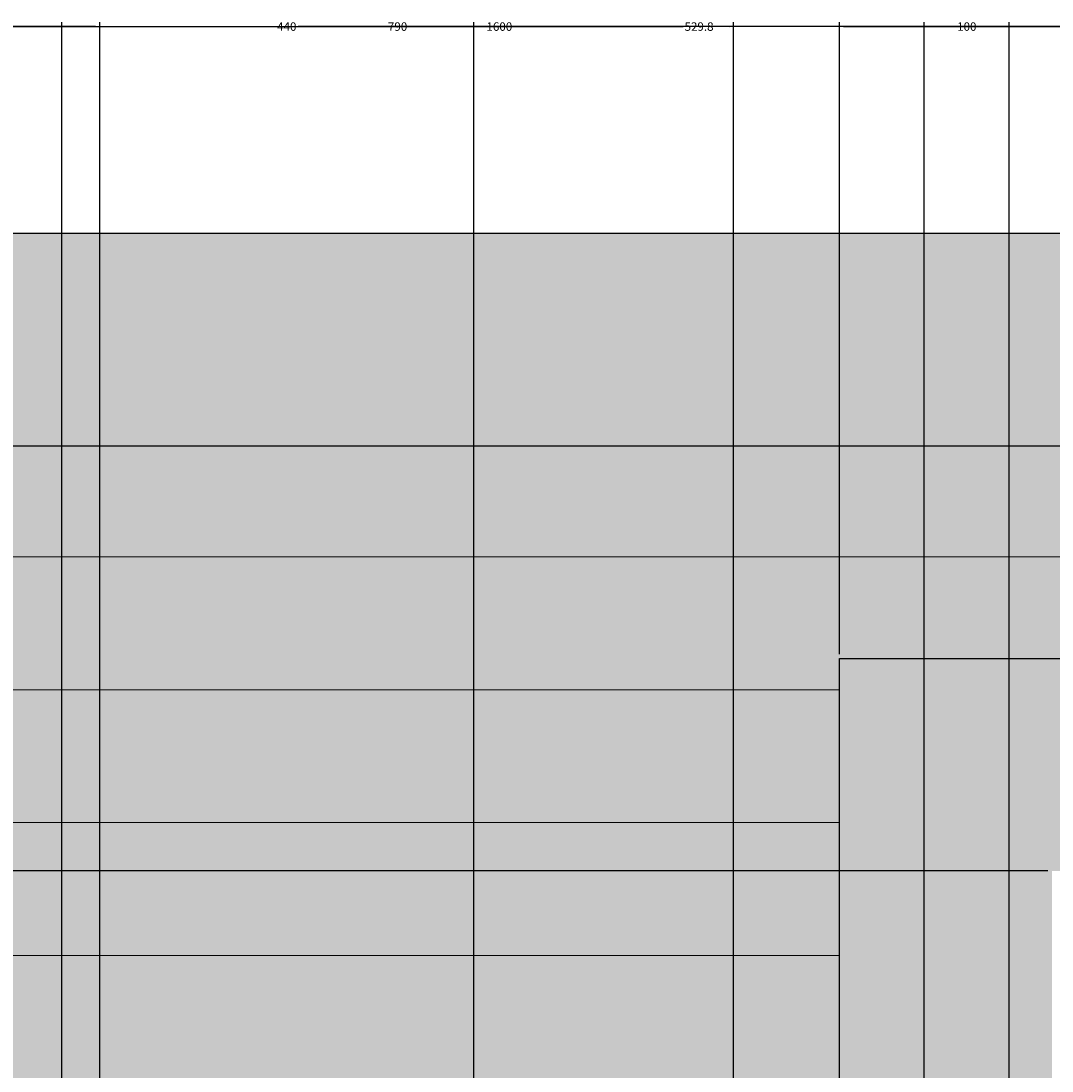
# Model space of a CAD drawing. Units: millimetres. Extents: x 2970 to 7764, y 2196 to 7505.
# Tile 12 of 13: x 4793 to 6006, y 6270 to 7505. Entities that reach past the tile are written whole.
import ezdxf

# ---------------------------------------------------------------- set-up
doc = ezdxf.new("R2010")
doc.units = ezdxf.units.MM
doc.header["$MEASUREMENT"] = 0
for name, color, linetype, lineweight in [('A-ANNO-DIMS', 2, 'Continuous', 18), ('A-ELEV', 7, 'Continuous', 25), ('A-ELEV-PATT', 8, 'Continuous', 13)]:
    doc.layers.add(name, color=color, linetype=linetype, lineweight=lineweight)
doc.styles.get("Standard").update_dxf_attribs({"font": 'arial.ttf'})
doc.dimstyles.get("Standard").update_dxf_attribs({"dimtxt": 10, "dimasz": 5, "dimexe": 5, "dimexo": 5, "dimgap": 2, "dimtad": 0, "dimtih": 1, "dimtoh": 1, "dimdec": 0, "dimzin": 0, "dimdsep": 46, "dimtxsty": 'Standard', "dimcen": 2, "dimadec": 0, "dimazin": 0, "dimtfac": 1, "dimtdec": 0, "dimtofl": 0, "dimtmove": 0, "dimatfit": 3, "dimfxl": 1, "dimtolj": 1, "dimtzin": 0, "dimarcsym": 0})

# ---------------------------------------------------------------- blocks, each defined once
blk = doc.blocks.new('*D17')
at = {"layer": 'A-ANNO-DIMS', "color": 0, "lineweight": -2, "transparency": 16777216}
for p, q in [((4555.5, 7010.8), (4555.5, 7503.8)), ((4560.5, 7498.8), (5339.1, 7498.8)), ((6150.5, 7498.8), (5371.9, 7498.8)), ((6155.5, 7010.8), (6155.5, 7503.8))]:
    blk.add_line(p, q, dxfattribs=at)
at = {"layer": 'A-ANNO-DIMS', "color": 0, "transparency": 16777216}
for points in [[(4560.5, 7499.6), (4560.5, 7498), (4555.5, 7498.8)], [(6150.5, 7499.6), (6150.5, 7498), (6155.5, 7498.8)]]:
    blk.add_solid(points, dxfattribs=at)
at = {"layer": 'Defpoints', "color": 0, "transparency": 16777216}
for p in [(6155.5, 7498.8), (4555.5, 7005.8), (6155.5, 7005.8)]:
    blk.add_point(p, dxfattribs=at)
at = {"layer": 'A-ANNO-DIMS', "color": 0, "transparency": 16777216, "insert": (5355.5, 7498.8), "char_height": 10, "attachment_point": 5}
blk.add_mtext('\\A1;1600', dxfattribs=at)
blk = doc.blocks.new('*D34')
at = {"layer": 'A-ANNO-DIMS', "color": 0, "lineweight": -2, "transparency": 16777216}
for p, q in [((4355.5, 4210.8), (4355.5, 7503.8)), ((4360.5, 7498.8), (4607.5, 7498.8)), ((4880.5, 7498.8), (4633.5, 7498.8)), ((4885.5, 4210.8), (4885.5, 7503.8))]:
    blk.add_line(p, q, dxfattribs=at)
at = {"layer": 'A-ANNO-DIMS', "color": 0, "transparency": 16777216}
for points in [[(4360.5, 7499.6), (4360.5, 7498), (4355.5, 7498.8)], [(4880.5, 7499.6), (4880.5, 7498), (4885.5, 7498.8)]]:
    blk.add_solid(points, dxfattribs=at)
at = {"layer": 'Defpoints', "color": 0, "transparency": 16777216}
for p in [(4885.5, 7498.8), (4355.5, 4205.8), (4885.5, 4205.8)]:
    blk.add_point(p, dxfattribs=at)
at = {"layer": 'A-ANNO-DIMS', "color": 0, "transparency": 16777216, "insert": (4620.5, 7498.8), "char_height": 10, "attachment_point": 5}
blk.add_mtext('\\A1;530', dxfattribs=at)
blk = doc.blocks.new('*D35')
at = {"layer": 'A-ANNO-DIMS', "color": 0, "lineweight": -2, "transparency": 16777216}
for p, q in [((4885.5, 4210.8), (4885.5, 7503.8)), ((4890.5, 7498.8), (5092.3, 7498.8)), ((5320.5, 7498.8), (5118.7, 7498.8)), ((5325.5, 4210.8), (5325.5, 7503.8))]:
    blk.add_line(p, q, dxfattribs=at)
at = {"layer": 'A-ANNO-DIMS', "color": 0, "transparency": 16777216}
for points in [[(4890.5, 7499.6), (4890.5, 7498), (4885.5, 7498.8)], [(5320.5, 7499.6), (5320.5, 7498), (5325.5, 7498.8)]]:
    blk.add_solid(points, dxfattribs=at)
at = {"layer": 'Defpoints', "color": 0, "transparency": 16777216}
for p in [(5325.5, 7498.8), (4885.5, 4205.8), (5325.5, 4205.8)]:
    blk.add_point(p, dxfattribs=at)
at = {"layer": 'A-ANNO-DIMS', "color": 0, "transparency": 16777216, "insert": (5105.5, 7498.8), "char_height": 10, "attachment_point": 5}
blk.add_mtext('\\A1;440', dxfattribs=at)
blk = doc.blocks.new('*D36')
at = {"layer": 'A-ANNO-DIMS', "color": 0, "lineweight": -2, "transparency": 16777216}
for p, q in [((5325.5, 4210.8), (5325.5, 7503.8)), ((5330.5, 7498.8), (5571.5, 7498.8)), ((5850.3, 7498.8), (5609.3, 7498.8)), ((5855.3, 4210.8), (5855.3, 7503.8))]:
    blk.add_line(p, q, dxfattribs=at)
at = {"layer": 'A-ANNO-DIMS', "color": 0, "transparency": 16777216}
for points in [[(5330.5, 7499.6), (5330.5, 7498), (5325.5, 7498.8)], [(5850.3, 7499.6), (5850.3, 7498), (5855.3, 7498.8)]]:
    blk.add_solid(points, dxfattribs=at)
at = {"layer": 'Defpoints', "color": 0, "transparency": 16777216}
for p in [(5855.3, 7498.8), (5325.5, 4205.8), (5855.3, 4205.8)]:
    blk.add_point(p, dxfattribs=at)
at = {"layer": 'A-ANNO-DIMS', "color": 0, "transparency": 16777216, "insert": (5590.4, 7498.8), "char_height": 10, "attachment_point": 5}
blk.add_mtext('\\A1;529.8', dxfattribs=at)
blk = doc.blocks.new('*D37')
at = {"layer": 'A-ANNO-DIMS', "color": 0, "lineweight": -2, "transparency": 16777216}
for p, q in [((5855.3, 4210.8), (5855.3, 7503.8)), ((5860.3, 7498.8), (5892.7, 7498.8)), ((5950.3, 7498.8), (5917.8, 7498.8)), ((5955.3, 4010.8), (5955.3, 7503.8))]:
    blk.add_line(p, q, dxfattribs=at)
at = {"layer": 'A-ANNO-DIMS', "color": 0, "transparency": 16777216}
for points in [[(5860.3, 7499.6), (5860.3, 7498), (5855.3, 7498.8)], [(5950.3, 7499.6), (5950.3, 7498), (5955.3, 7498.8)]]:
    blk.add_solid(points, dxfattribs=at)
at = {"layer": 'Defpoints', "color": 0, "transparency": 16777216}
for p in [(5955.3, 7498.8), (5855.3, 4205.8), (5955.3, 4005.8)]:
    blk.add_point(p, dxfattribs=at)
at = {"layer": 'A-ANNO-DIMS', "color": 0, "transparency": 16777216, "insert": (5905.3, 7498.8), "char_height": 10, "attachment_point": 5}
blk.add_mtext('\\A1;100', dxfattribs=at)
blk = doc.blocks.new('*D39')
at = {"layer": 'A-ANNO-DIMS', "color": 0, "lineweight": -2, "transparency": 16777216}
for p, q in [((5955.3, 4010.8), (5955.3, 7503.8)), ((5960.3, 7498.8), (6117.2, 7498.8)), ((6300.3, 7498.8), (6143.3, 7498.8)), ((6305.3, 4010.8), (6305.3, 7503.8))]:
    blk.add_line(p, q, dxfattribs=at)
at = {"layer": 'A-ANNO-DIMS', "color": 0, "transparency": 16777216}
for points in [[(5960.3, 7499.6), (5960.3, 7498), (5955.3, 7498.8)], [(6300.3, 7499.6), (6300.3, 7498), (6305.3, 7498.8)]]:
    blk.add_solid(points, dxfattribs=at)
at = {"layer": 'Defpoints', "color": 0, "transparency": 16777216}
for p in [(6305.3, 7498.8), (5955.3, 4005.8), (6305.3, 4005.8)]:
    blk.add_point(p, dxfattribs=at)
at = {"layer": 'A-ANNO-DIMS', "color": 0, "transparency": 16777216, "insert": (6130.3, 7498.8), "char_height": 10, "attachment_point": 5}
blk.add_mtext('\\A1;350', dxfattribs=at)
blk = doc.blocks.new('*D65')
at = {"layer": 'A-ANNO-DIMS', "color": 0, "lineweight": -2, "transparency": 16777216}
for p, q in [((4840.8, 6242.5), (4840.8, 7503.8)), ((4845.8, 7498.8), (5222.8, 7498.8)), ((5625.8, 7498.8), (5248.8, 7498.8)), ((5630.8, 6242.5), (5630.8, 7503.8))]:
    blk.add_line(p, q, dxfattribs=at)
at = {"layer": 'A-ANNO-DIMS', "color": 0, "transparency": 16777216}
for points in [[(4845.8, 7499.6), (4845.8, 7498), (4840.8, 7498.8)], [(5625.8, 7499.6), (5625.8, 7498), (5630.8, 7498.8)]]:
    blk.add_solid(points, dxfattribs=at)
at = {"layer": 'Defpoints', "color": 0, "transparency": 16777216}
for p in [(5630.8, 7498.8), (4840.8, 6237.5), (5630.8, 6237.5)]:
    blk.add_point(p, dxfattribs=at)
at = {"layer": 'A-ANNO-DIMS', "color": 0, "transparency": 16777216, "insert": (5235.8, 7498.8), "char_height": 10, "attachment_point": 5}
blk.add_mtext('\\A1;790', dxfattribs=at)
blk = doc.blocks.new('*D67')
at = {"layer": 'A-ANNO-DIMS', "color": 0, "lineweight": -2, "transparency": 16777216}
for p, q in [((5755.5, 6760.8), (5755.5, 7503.8)), ((5760.5, 7498.8), (6564.1, 7498.8)), ((7400.5, 7498.8), (6596.9, 7498.8)), ((7405.5, 6760.8), (7405.5, 7503.8))]:
    blk.add_line(p, q, dxfattribs=at)
at = {"layer": 'A-ANNO-DIMS', "color": 0, "transparency": 16777216}
for points in [[(5760.5, 7499.6), (5760.5, 7498), (5755.5, 7498.8)], [(7400.5, 7499.6), (7400.5, 7498), (7405.5, 7498.8)]]:
    blk.add_solid(points, dxfattribs=at)
at = {"layer": 'Defpoints', "color": 0, "transparency": 16777216}
for p in [(7405.5, 7498.8), (5755.5, 6755.8), (7405.5, 6755.8)]:
    blk.add_point(p, dxfattribs=at)
at = {"layer": 'A-ANNO-DIMS', "color": 0, "transparency": 16777216, "insert": (6580.5, 7498.8), "char_height": 10, "attachment_point": 5}
blk.add_mtext('\\A1;1650', dxfattribs=at)
blk = doc.blocks.new('*D82')
at = {"layer": 'A-ANNO-DIMS', "color": 0, "lineweight": -2, "transparency": 16777216}
for p, q in [((6000.5, 6505.8), (2982.5, 6505.8)), ((2987.5, 6500.8), (2987.5, 6375.4)), ((2987.5, 6235.8), (2987.5, 6361.2)), ((6000.5, 6230.8), (2982.5, 6230.8))]:
    blk.add_line(p, q, dxfattribs=at)
at = {"layer": 'A-ANNO-DIMS', "color": 0, "transparency": 16777216}
for points in [[(2986.7, 6500.8), (2988.3, 6500.8), (2987.5, 6505.8)], [(2986.7, 6235.8), (2988.3, 6235.8), (2987.5, 6230.8)]]:
    blk.add_solid(points, dxfattribs=at)
at = {"layer": 'Defpoints', "color": 0, "transparency": 16777216}
for p in [(2987.5, 6505.8), (6005.5, 6505.8), (6005.5, 6230.8)]:
    blk.add_point(p, dxfattribs=at)
at = {"layer": 'A-ANNO-DIMS', "color": 0, "transparency": 16777216, "insert": (2987.5, 6368.3), "char_height": 10, "attachment_point": 5}
blk.add_mtext('\\A1;275', dxfattribs=at)

msp = doc.modelspace()

# ---------------------------------------------------------------- hatches: boundary and pattern name
at = {"layer": 'A-ELEV-PATT'}
h = msp.add_hatch(color=256, dxfattribs=at)
h.dxf.hatch_style = 1
h.paths.add_polyline_path([(6405.5, 7255.789), (4305.5, 7255.789), (4305.5, 6505.789), (3730.5, 6505.789), (3730.5, 4205.789), (3730.5, 2945.789), (3730.5, 2895.789), (3830.5, 2895.789), (3830.5, 4205.789), (3830.5, 6405.789), (4405.5, 6405.789), (4405.5, 4205.789), (6905.5, 4205.789), (6905.5, 2945.789), (6905.5, 2845.789), (7155.5, 2845.789), (7155.5, 2945.789), (7155.5, 4205.789), (7155.5, 4455.789), (4555.5, 4455.789), (4555.5, 6505.789), (4555.5, 7005.789), (6155.5, 7005.789), (6155.5, 6755.789), (6405.5, 6755.789)])
h.paths.add_polyline_path([(7405.5, 6755.789), (6155.5, 6755.789), (5755.5, 6755.789), (5755.5, 5005.789), (7405.5, 5005.789)])
h.paths.add_polyline_path([(7155.5, 6505.789), (7155.5, 5255.789), (6005.5, 5255.789), (6005.5, 6505.789)], flags=16)
h.paths.add_polyline_path([(6105.5, 5520.789), (6105.5, 6055.789), (6455.5, 6055.789), (6455.5, 5520.789), (6655.5, 5520.789), (6655.5, 5605.789), (6655.5, 5955.789), (6955.5, 5955.789), (6955.5, 5605.789), (6955.5, 5520.789)], flags=0)
h.paths.add_polyline_path([(6425.5, 5755.789), (6425.5, 5655.789), (6425.5, 5555.789), (6405.5, 5555.789), (6405.5, 5755.789)], flags=0)
h.paths.add_polyline_path([(6955.5, 5505.789), (6955.5, 5405.789), (6655.5, 5405.789), (6655.5, 5505.789)], flags=0)
h = msp.add_hatch(color=256, dxfattribs=at)
h.set_gradient(color1=(147, 149, 152), color2=(199, 200, 202), name='CURVED')
h.paths.add_polyline_path([(6955.5, 4455.789), (6955.5, 5005.789), (5755.5, 5005.789), (5755.5, 6755.789), (6155.5, 6755.789), (6155.5, 7005.789), (4555.5, 7005.789), (4555.5, 6505.789), (4555.5, 4455.789)])
h.paths.add_polyline_path([(5015.81, 5462.49), (5015.81, 6062.49), (5455.81, 6062.49), (5455.81, 5462.49)], flags=16)
h.paths.add_polyline_path([(5035.81, 5482.49), (5035.81, 6042.49), (5155.81, 6042.49), (5155.81, 5482.49)], flags=0)
h.paths.add_polyline_path([(5175.81, 5482.49), (5175.81, 6042.49), (5295.81, 6042.49), (5295.81, 5482.49)], flags=0)
h.paths.add_polyline_path([(5315.81, 5482.49), (5315.81, 6042.49), (5435.81, 6042.49), (5435.81, 5482.49)], flags=0)
h.paths.add_polyline_path([(4865.81, 6162.49), (4865.81, 6212.49), (4840.81, 6212.49), (4840.81, 6237.49), (5630.81, 6237.49), (5630.81, 6212.49), (5605.81, 6212.49), (5605.81, 6162.49), (5015.81, 6162.49)], flags=16)
h = msp.add_hatch(dxfattribs=at)
h.set_pattern_fill('ANSI31', color=256, scale=1250, angle=135, style=0)
h.paths.add_polyline_path([(5755.5, 6755.789), (6155.5, 6755.789), (6155.5, 7005.789), (4555.5, 7005.789), (4555.5, 6505.789), (4555.5, 4455.789), (6955.5, 4455.789), (6955.5, 5005.789), (5755.5, 5005.789)])
h.paths.add_polyline_path([(5015.81, 5462.49), (5015.81, 6062.49), (5455.81, 6062.49), (5455.81, 5462.49)], flags=16)
h.paths.add_polyline_path([(5035.81, 5482.49), (5035.81, 6042.49), (5155.81, 6042.49), (5155.81, 5482.49)], flags=0)
h.paths.add_polyline_path([(5175.81, 5482.49), (5175.81, 6042.49), (5295.81, 6042.49), (5295.81, 5482.49)], flags=0)
h.paths.add_polyline_path([(5315.81, 5482.49), (5315.81, 6042.49), (5435.81, 6042.49), (5435.81, 5482.49)], flags=0)
h.paths.add_polyline_path([(4865.81, 6162.49), (4865.81, 6212.49), (4840.81, 6212.49), (4840.81, 6237.49), (5630.81, 6237.49), (5630.81, 6212.49), (5605.81, 6212.49), (5605.81, 6162.49), (5015.81, 6162.49)], flags=16)

# ---------------------------------------------------------------- linework, layer by layer
at = {"layer": 'A-ELEV'}
for p, q in [((4305.5, 7255.789), (6405.5, 7255.789)), ((4555.5, 7005.789), (6155.5, 7005.789)), ((5755.5, 5005.789), (5755.5, 6755.789)), ((5755.5, 6755.789), (6155.5, 6755.789))]:
    msp.add_line(p, q, dxfattribs=at)

# ---------------------------------------------------------------- dimensions: what is measured, and where the dimension line sits
at = {"layer": 'A-ANNO-DIMS'}
for base, p1, p2, override, picture, middle in [((4885.5, 7498.789), (4355.5, 4205.789), (4885.5, 4205.789), {"dimdec": 0, "dimlfac": 1, "dimrnd": 0, "dimzin": 0, "dimdsep": 46, "dimlunit": 2}, '*D34', (4620.5, 7498.789)), ((6155.5, 7498.789), (4555.5, 7005.789), (6155.5, 7005.789), {"dimdec": 0, "dimlfac": 1, "dimrnd": 0, "dimzin": 0, "dimdsep": 46, "dimlunit": 2}, '*D17', (5355.5, 7498.789)), ((5630.81, 7498.789), (4840.81, 6237.49), (5630.81, 6237.49), {"dimdec": 0, "dimlfac": 1, "dimrnd": 0, "dimzin": 0, "dimdsep": 46, "dimlunit": 2}, '*D65', (5235.81, 7498.789)), ((5325.5, 7498.789), (4885.5, 4205.789), (5325.5, 4205.789), {"dimdec": 0, "dimlfac": 1, "dimrnd": 0, "dimzin": 0, "dimdsep": 46, "dimlunit": 2}, '*D35', (5105.5, 7498.789)), ((5855.271, 7498.789), (5325.5, 4205.789), (5855.271, 4205.789), {"dimdec": 1, "dimlfac": 1, "dimrnd": 0, "dimzin": 0, "dimdsep": 46, "dimlunit": 2}, '*D36', (5590.386, 7498.789)), ((7405.5, 7498.789), (5755.5, 6755.789), (7405.5, 6755.789), {"dimdec": 0, "dimlfac": 1, "dimrnd": 0, "dimzin": 0, "dimdsep": 46, "dimlunit": 2}, '*D67', (6580.5, 7498.789)), ((5955.271, 7498.789), (5855.271, 4205.789), (5955.271, 4005.789), {"dimdec": 0, "dimlfac": 1, "dimrnd": 0, "dimzin": 0, "dimdsep": 46, "dimlunit": 2}, '*D37', (5905.271, 7498.789)), ((6305.271, 7498.789), (5955.271, 4005.789), (6305.271, 4005.789), {"dimdec": 0, "dimlfac": 1, "dimrnd": 0, "dimzin": 0, "dimdsep": 46, "dimlunit": 2}, '*D39', (6130.271, 7498.789))]:
    dim = msp.add_linear_dim(base=base, p1=p1, p2=p2, dimstyle='Standard', override=override, dxfattribs=at)
    dim.commit()
    dim.dimension.update_dxf_attribs({"geometry": picture, "text_midpoint": middle})
dim = msp.add_linear_dim(base=(2987.5, 6505.789), p1=(6005.5, 6230.789), p2=(6005.5, 6505.789), angle=90, dimstyle='Standard', override={"dimdec": 0, "dimlfac": 1, "dimrnd": 0, "dimzin": 0, "dimdsep": 46, "dimlunit": 2}, dxfattribs=at)
dim.commit()
dim.dimension.update_dxf_attribs({"geometry": '*D82', "text_midpoint": (2987.5, 6368.289)})

doc.saveas('drawing.dxf')
